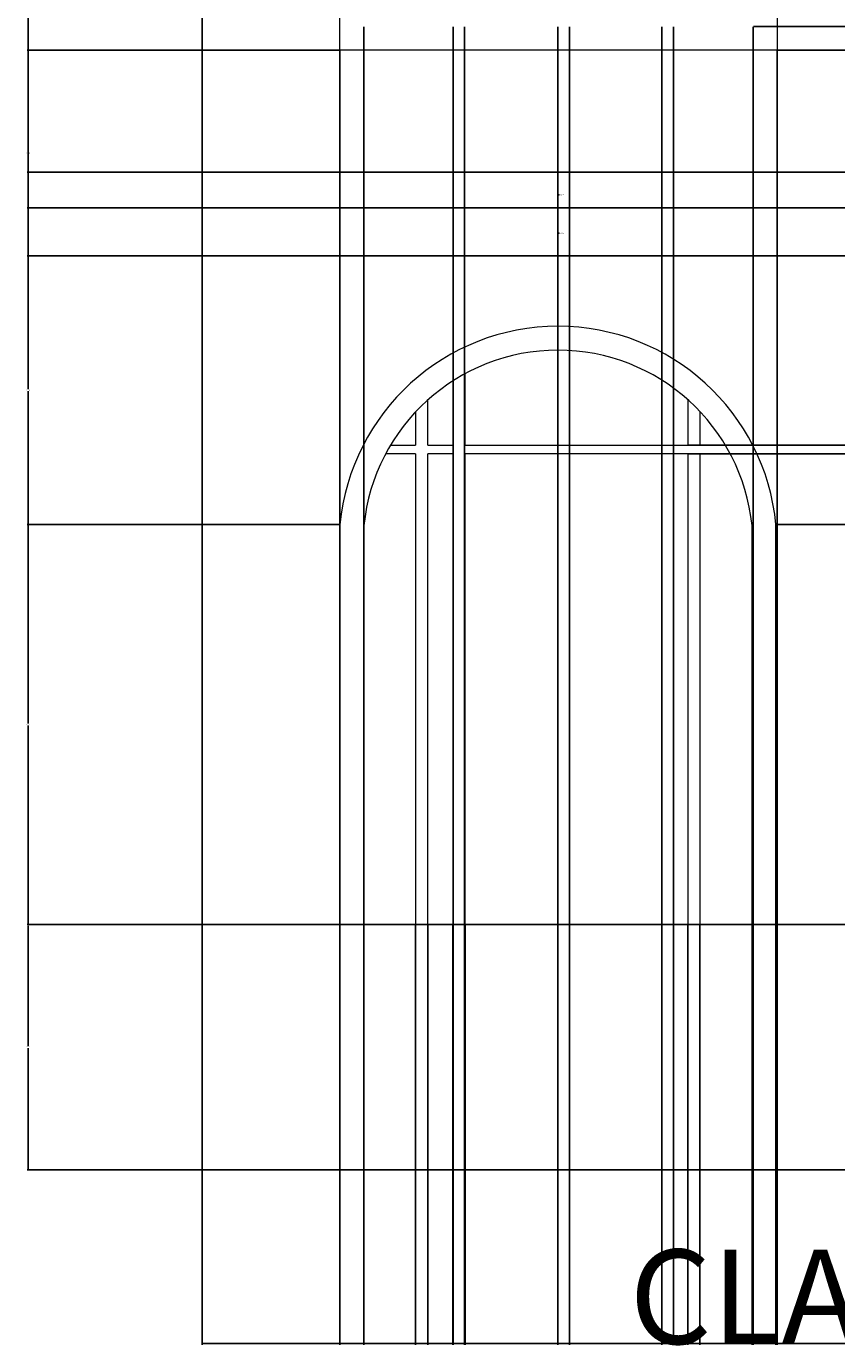
# Model space of a CAD drawing. Units: inches. Extents: x -14 to 375, y -86 to 549.
# Tile 1 of 12: x -14 to 122, y -65 to 156. Entities that reach past the tile are written whole.
import ezdxf

# ---------------------------------------------------------------- set-up
doc = ezdxf.new("R2010")
doc.units = ezdxf.units.IN
doc.header["$MEASUREMENT"] = 0
for name, color, linetype, lineweight in [('A-ANNO-DIMS', 2, 'Continuous', 18), ('A-ANNO-TEXT', 7, 'Continuous', 25), ('A-ELEV', 7, 'Continuous', 25), ('A-GLAZ', 4, 'Continuous', 18)]:
    doc.layers.add(name, color=color, linetype=linetype, lineweight=lineweight)
doc.styles.get("Standard").update_dxf_attribs({"font": 'arial.ttf'})
doc.dimstyles.get("Standard").update_dxf_attribs({"dimtxt": 0.18, "dimasz": 0.18, "dimexe": 0.18, "dimexo": 0.0625, "dimgap": 0.09, "dimtad": 0, "dimtih": 1, "dimtoh": 1, "dimdec": 4, "dimzin": 0, "dimdsep": 46, "dimtxsty": 'Standard', "dimcen": 0.09, "dimadec": 0, "dimazin": 0, "dimtfac": 1, "dimtdec": 4, "dimtofl": 0, "dimtmove": 0, "dimatfit": 3, "dimfxl": 1, "dimtolj": 1, "dimtzin": 0, "dimarcsym": 0})

# ---------------------------------------------------------------- blocks, each defined once
blk = doc.blocks.new('*D4')
at = {"layer": 'A-ANNO-DIMS', "color": 0, "lineweight": -2, "transparency": 16777216}
for p, q in [((15.4, -35.17), (15.4, -64.39)), ((345.26, -35.17), (345.26, -64.39)), ((15.58, -64.21), (179.87, -64.21)), ((345.08, -64.21), (180.8, -64.21))]:
    blk.add_line(p, q, dxfattribs=at)
at = {"layer": 'A-ANNO-DIMS', "color": 0, "transparency": 16777216}
for points in [[(15.58, -64.18), (15.58, -64.24), (15.4, -64.21)], [(345.08, -64.18), (345.08, -64.24), (345.26, -64.21)]]:
    blk.add_solid(points, dxfattribs=at)
at = {"layer": 'Defpoints', "color": 0, "transparency": 16777216}
for p in [(15.4, -35.11), (345.26, -35.11), (345.26, -64.21)]:
    blk.add_point(p, dxfattribs=at)
at = {"layer": 'A-ANNO-DIMS', "color": 0, "transparency": 16777216, "insert": (180.33, -64.21), "char_height": 0.18, "attachment_point": 5}
blk.add_mtext('\\A1;329.86', dxfattribs=at)
blk = doc.blocks.new('*D11')
at = {"layer": 'A-ANNO-DIMS', "color": 0, "lineweight": -2, "transparency": 16777216}
for p, q in [((38.44, 5.96), (-13.88, 5.96)), ((-13.7, 5.78), (-13.7, -14.39)), ((-13.7, -34.93), (-13.7, -14.76)), ((15.34, -35.11), (-13.88, -35.11))]:
    blk.add_line(p, q, dxfattribs=at)
at = {"layer": 'A-ANNO-DIMS', "color": 0, "transparency": 16777216}
for points in [[(-13.73, 5.78), (-13.67, 5.78), (-13.7, 5.96)], [(-13.73, -34.93), (-13.67, -34.93), (-13.7, -35.11)]]:
    blk.add_solid(points, dxfattribs=at)
at = {"layer": 'Defpoints', "color": 0, "transparency": 16777216}
for p in [(-13.7, 5.96), (38.5, 5.96), (15.4, -35.11)]:
    blk.add_point(p, dxfattribs=at)
at = {"layer": 'A-ANNO-DIMS', "color": 0, "transparency": 16777216, "insert": (-13.7, -14.58), "char_height": 0.18, "attachment_point": 5}
blk.add_mtext('\\A1;41.07', dxfattribs=at)
blk = doc.blocks.new('*D12')
at = {"layer": 'A-ANNO-DIMS', "color": 0, "lineweight": -2, "transparency": 16777216}
for p, q in [((38.44, 72.97), (-13.88, 72.97)), ((-13.7, 72.79), (-13.7, 39.65)), ((-13.7, 6.14), (-13.7, 39.28)), ((38.44, 5.96), (-13.88, 5.96))]:
    blk.add_line(p, q, dxfattribs=at)
at = {"layer": 'A-ANNO-DIMS', "color": 0, "transparency": 16777216}
for points in [[(-13.73, 72.79), (-13.67, 72.79), (-13.7, 72.97)], [(-13.73, 6.14), (-13.67, 6.14), (-13.7, 5.96)]]:
    blk.add_solid(points, dxfattribs=at)
at = {"layer": 'Defpoints', "color": 0, "transparency": 16777216}
for p in [(-13.7, 72.97), (38.5, 72.97), (38.5, 5.96)]:
    blk.add_point(p, dxfattribs=at)
at = {"layer": 'A-ANNO-DIMS', "color": 0, "transparency": 16777216, "insert": (-13.7, 39.46), "char_height": 0.18, "attachment_point": 5}
blk.add_mtext('\\A1;67.01', dxfattribs=at)
blk = doc.blocks.new('*D13')
at = {"layer": 'A-ANNO-DIMS', "color": 0, "lineweight": -2, "transparency": 16777216}
for p, q in [((134.17, 117.96), (-13.88, 117.96)), ((-13.7, 117.78), (-13.7, 95.65)), ((-13.7, 73.15), (-13.7, 95.28)), ((38.44, 72.97), (-13.88, 72.97))]:
    blk.add_line(p, q, dxfattribs=at)
at = {"layer": 'A-ANNO-DIMS', "color": 0, "transparency": 16777216}
for points in [[(-13.73, 117.78), (-13.67, 117.78), (-13.7, 117.96)], [(-13.73, 73.15), (-13.67, 73.15), (-13.7, 72.97)]]:
    blk.add_solid(points, dxfattribs=at)
at = {"layer": 'Defpoints', "color": 0, "transparency": 16777216}
for p in [(-13.7, 117.96), (134.23, 117.96), (38.5, 72.97)]:
    blk.add_point(p, dxfattribs=at)
at = {"layer": 'A-ANNO-DIMS', "color": 0, "transparency": 16777216, "insert": (-13.7, 95.46), "char_height": 0.18, "attachment_point": 5}
blk.add_mtext('\\A1;44.99', dxfattribs=at)
blk = doc.blocks.new('*D14')
at = {"layer": 'A-ANNO-DIMS', "color": 0, "lineweight": -2, "transparency": 16777216}
for p, q in [((38.44, 152.38), (-13.88, 152.38)), ((-13.7, 152.2), (-13.7, 135.35)), ((-13.7, 118.14), (-13.7, 134.99)), ((134.17, 117.96), (-13.88, 117.96))]:
    blk.add_line(p, q, dxfattribs=at)
at = {"layer": 'A-ANNO-DIMS', "color": 0, "transparency": 16777216}
for points in [[(-13.73, 152.2), (-13.67, 152.2), (-13.7, 152.38)], [(-13.73, 118.14), (-13.67, 118.14), (-13.7, 117.96)]]:
    blk.add_solid(points, dxfattribs=at)
at = {"layer": 'Defpoints', "color": 0, "transparency": 16777216}
for p in [(-13.7, 152.38), (38.5, 152.38), (134.23, 117.96)]:
    blk.add_point(p, dxfattribs=at)
at = {"layer": 'A-ANNO-DIMS', "color": 0, "transparency": 16777216, "insert": (-13.7, 135.17), "char_height": 0.18, "attachment_point": 5}
blk.add_mtext('\\A1;34.42', dxfattribs=at)
blk = doc.blocks.new('*D15')
at = {"layer": 'A-ANNO-DIMS', "color": 0, "lineweight": -2, "transparency": 16777216}
for p, q in [((134.17, 187.85), (-13.88, 187.85)), ((-13.7, 187.67), (-13.7, 170.29)), ((-13.7, 152.56), (-13.7, 169.93)), ((38.44, 152.38), (-13.88, 152.38))]:
    blk.add_line(p, q, dxfattribs=at)
at = {"layer": 'A-ANNO-DIMS', "color": 0, "transparency": 16777216}
for points in [[(-13.73, 187.67), (-13.67, 187.67), (-13.7, 187.85)], [(-13.73, 152.56), (-13.67, 152.56), (-13.7, 152.38)]]:
    blk.add_solid(points, dxfattribs=at)
at = {"layer": 'Defpoints', "color": 0, "transparency": 16777216}
for p in [(-13.7, 187.85), (134.23, 187.85), (38.5, 152.38)]:
    blk.add_point(p, dxfattribs=at)
at = {"layer": 'A-ANNO-DIMS', "color": 0, "transparency": 16777216, "insert": (-13.7, 170.11), "char_height": 0.18, "attachment_point": 5}
blk.add_mtext('\\A1;35.47', dxfattribs=at)
blk = doc.blocks.new('*D19')
at = {"layer": 'A-ANNO-DIMS', "color": 0, "lineweight": -2, "transparency": 16777216}
for p, q in [((42.5, 156.31), (42.5, -64.39)), ((38.5, 152.31), (38.5, -64.39)), ((38.68, -64.21), (40.35, -64.21)), ((42.32, -64.21), (40.66, -64.21))]:
    blk.add_line(p, q, dxfattribs=at)
at = {"layer": 'A-ANNO-DIMS', "color": 0, "transparency": 16777216}
for points in [[(38.68, -64.18), (38.68, -64.24), (38.5, -64.21)], [(42.32, -64.18), (42.32, -64.24), (42.5, -64.21)]]:
    blk.add_solid(points, dxfattribs=at)
at = {"layer": 'Defpoints', "color": 0, "transparency": 16777216}
for p in [(42.5, 156.38), (38.5, 152.38), (42.5, -64.21)]:
    blk.add_point(p, dxfattribs=at)
at = {"layer": 'A-ANNO-DIMS', "color": 0, "transparency": 16777216, "insert": (40.5, -64.21), "char_height": 0.18, "attachment_point": 5}
blk.add_mtext('\\A1;4', dxfattribs=at)
blk = doc.blocks.new('*D20')
at = {"layer": 'A-ANNO-DIMS', "color": 0, "lineweight": -2, "transparency": 16777216}
for p, q in [((42.5, 156.31), (42.5, -64.39)), ((57.44, 156.31), (57.44, -64.39)), ((42.68, -64.21), (49.52, -64.21)), ((57.26, -64.21), (50.43, -64.21))]:
    blk.add_line(p, q, dxfattribs=at)
at = {"layer": 'A-ANNO-DIMS', "color": 0, "transparency": 16777216}
for points in [[(42.68, -64.18), (42.68, -64.24), (42.5, -64.21)], [(57.26, -64.18), (57.26, -64.24), (57.44, -64.21)]]:
    blk.add_solid(points, dxfattribs=at)
at = {"layer": 'Defpoints', "color": 0, "transparency": 16777216}
for p in [(42.5, 156.38), (57.44, 156.38), (57.44, -64.21)]:
    blk.add_point(p, dxfattribs=at)
at = {"layer": 'A-ANNO-DIMS', "color": 0, "transparency": 16777216, "insert": (49.97, -64.21), "char_height": 0.18, "attachment_point": 5}
blk.add_mtext('\\A1;14.938', dxfattribs=at)
blk = doc.blocks.new('*D21')
at = {"layer": 'A-ANNO-DIMS', "color": 0, "lineweight": -2, "transparency": 16777216}
for p, q in [((57.44, 156.31), (57.44, -64.39)), ((59.36, 156.31), (59.36, -64.39)), ((57.62, -64.21), (58.09, -64.21)), ((59.18, -64.21), (58.72, -64.21))]:
    blk.add_line(p, q, dxfattribs=at)
at = {"layer": 'A-ANNO-DIMS', "color": 0, "transparency": 16777216}
for points in [[(57.62, -64.18), (57.62, -64.24), (57.44, -64.21)], [(59.18, -64.18), (59.18, -64.24), (59.36, -64.21)]]:
    blk.add_solid(points, dxfattribs=at)
at = {"layer": 'Defpoints', "color": 0, "transparency": 16777216}
for p in [(57.44, 156.38), (59.36, 156.38), (59.36, -64.21)]:
    blk.add_point(p, dxfattribs=at)
at = {"layer": 'A-ANNO-DIMS', "color": 0, "transparency": 16777216, "insert": (58.4, -64.21), "char_height": 0.18, "attachment_point": 5}
blk.add_mtext('\\A1;1.92', dxfattribs=at)
blk = doc.blocks.new('*D22')
at = {"layer": 'A-ANNO-DIMS', "color": 0, "lineweight": -2, "transparency": 16777216}
for p, q in [((59.36, 156.31), (59.36, -64.39)), ((75, 156.31), (75, -64.39)), ((59.54, -64.21), (66.73, -64.21)), ((74.82, -64.21), (67.64, -64.21))]:
    blk.add_line(p, q, dxfattribs=at)
at = {"layer": 'A-ANNO-DIMS', "color": 0, "transparency": 16777216}
for points in [[(59.54, -64.18), (59.54, -64.24), (59.36, -64.21)], [(74.82, -64.18), (74.82, -64.24), (75, -64.21)]]:
    blk.add_solid(points, dxfattribs=at)
at = {"layer": 'Defpoints', "color": 0, "transparency": 16777216}
for p in [(59.36, 156.38), (75, 156.38), (75, -64.21)]:
    blk.add_point(p, dxfattribs=at)
at = {"layer": 'A-ANNO-DIMS', "color": 0, "transparency": 16777216, "insert": (67.18, -64.21), "char_height": 0.18, "attachment_point": 5}
blk.add_mtext('\\A1;15.637', dxfattribs=at)
blk = doc.blocks.new('*D23')
at = {"layer": 'A-ANNO-DIMS', "color": 0, "lineweight": -2, "transparency": 16777216}
for p, q in [((75, 156.31), (75, -64.39)), ((76.92, 156.31), (76.92, -64.39)), ((75.18, -64.21), (75.65, -64.21)), ((76.74, -64.21), (76.28, -64.21))]:
    blk.add_line(p, q, dxfattribs=at)
at = {"layer": 'A-ANNO-DIMS', "color": 0, "transparency": 16777216}
for points in [[(75.18, -64.18), (75.18, -64.24), (75, -64.21)], [(76.74, -64.18), (76.74, -64.24), (76.92, -64.21)]]:
    blk.add_solid(points, dxfattribs=at)
at = {"layer": 'Defpoints', "color": 0, "transparency": 16777216}
for p in [(75, 156.38), (76.92, 156.38), (76.92, -64.21)]:
    blk.add_point(p, dxfattribs=at)
at = {"layer": 'A-ANNO-DIMS', "color": 0, "transparency": 16777216, "insert": (75.96, -64.21), "char_height": 0.18, "attachment_point": 5}
blk.add_mtext('\\A1;1.92', dxfattribs=at)
blk = doc.blocks.new('*D24')
at = {"layer": 'A-ANNO-DIMS', "color": 0, "lineweight": -2, "transparency": 16777216}
for p, q in [((76.92, 156.31), (76.92, -64.39)), ((92.4, 156.31), (92.4, -64.39)), ((77.1, -64.21), (84.2, -64.21)), ((92.22, -64.21), (85.12, -64.21))]:
    blk.add_line(p, q, dxfattribs=at)
at = {"layer": 'A-ANNO-DIMS', "color": 0, "transparency": 16777216}
for points in [[(77.1, -64.18), (77.1, -64.24), (76.92, -64.21)], [(92.22, -64.18), (92.22, -64.24), (92.4, -64.21)]]:
    blk.add_solid(points, dxfattribs=at)
at = {"layer": 'Defpoints', "color": 0, "transparency": 16777216}
for p in [(76.92, 156.38), (92.4, 156.38), (92.4, -64.21)]:
    blk.add_point(p, dxfattribs=at)
at = {"layer": 'A-ANNO-DIMS', "color": 0, "transparency": 16777216, "insert": (84.66, -64.21), "char_height": 0.18, "attachment_point": 5}
blk.add_mtext('\\A1;15.473', dxfattribs=at)
blk = doc.blocks.new('*D25')
at = {"layer": 'A-ANNO-DIMS', "color": 0, "lineweight": -2, "transparency": 16777216}
for p, q in [((92.4, 156.31), (92.4, -64.39)), ((94.32, 156.31), (94.32, -64.39)), ((92.58, -64.21), (93.04, -64.21)), ((94.14, -64.21), (93.67, -64.21))]:
    blk.add_line(p, q, dxfattribs=at)
at = {"layer": 'A-ANNO-DIMS', "color": 0, "transparency": 16777216}
for points in [[(92.58, -64.18), (92.58, -64.24), (92.4, -64.21)], [(94.14, -64.18), (94.14, -64.24), (94.32, -64.21)]]:
    blk.add_solid(points, dxfattribs=at)
at = {"layer": 'Defpoints', "color": 0, "transparency": 16777216}
for p in [(92.4, 156.38), (94.32, 156.38), (94.32, -64.21)]:
    blk.add_point(p, dxfattribs=at)
at = {"layer": 'A-ANNO-DIMS', "color": 0, "transparency": 16777216, "insert": (93.36, -64.21), "char_height": 0.18, "attachment_point": 5}
blk.add_mtext('\\A1;1.92', dxfattribs=at)
blk = doc.blocks.new('*D26')
at = {"layer": 'A-ANNO-DIMS', "color": 0, "lineweight": -2, "transparency": 16777216}
for p, q in [((94.32, 156.31), (94.32, -64.39)), ((107.7, 156.31), (107.7, -64.39)), ((94.5, -64.21), (100.56, -64.21)), ((107.52, -64.21), (101.47, -64.21))]:
    blk.add_line(p, q, dxfattribs=at)
at = {"layer": 'A-ANNO-DIMS', "color": 0, "transparency": 16777216}
for points in [[(94.5, -64.18), (94.5, -64.24), (94.32, -64.21)], [(107.52, -64.18), (107.52, -64.24), (107.7, -64.21)]]:
    blk.add_solid(points, dxfattribs=at)
at = {"layer": 'Defpoints', "color": 0, "transparency": 16777216}
for p in [(94.32, 156.38), (107.7, 156.38), (107.7, -64.21)]:
    blk.add_point(p, dxfattribs=at)
at = {"layer": 'A-ANNO-DIMS', "color": 0, "transparency": 16777216, "insert": (101.01, -64.21), "char_height": 0.18, "attachment_point": 5}
blk.add_mtext('\\A1;13.383', dxfattribs=at)
blk = doc.blocks.new('*D27')
at = {"layer": 'A-ANNO-DIMS', "color": 0, "lineweight": -2, "transparency": 16777216}
for p, q in [((107.7, 156.31), (107.7, -64.39)), ((111.7, 152.31), (111.7, -64.39)), ((107.88, -64.21), (109.55, -64.21)), ((111.52, -64.21), (109.85, -64.21))]:
    blk.add_line(p, q, dxfattribs=at)
at = {"layer": 'A-ANNO-DIMS', "color": 0, "transparency": 16777216}
for points in [[(107.88, -64.18), (107.88, -64.24), (107.7, -64.21)], [(111.52, -64.18), (111.52, -64.24), (111.7, -64.21)]]:
    blk.add_solid(points, dxfattribs=at)
at = {"layer": 'Defpoints', "color": 0, "transparency": 16777216}
for p in [(107.7, 156.38), (111.7, 152.38), (111.7, -64.21)]:
    blk.add_point(p, dxfattribs=at)
at = {"layer": 'A-ANNO-DIMS', "color": 0, "transparency": 16777216, "insert": (109.7, -64.21), "char_height": 0.18, "attachment_point": 5}
blk.add_mtext('\\A1;4', dxfattribs=at)
blk = doc.blocks.new('*D28')
at = {"layer": 'A-ANNO-DIMS', "color": 0, "lineweight": -2, "transparency": 16777216}
for p, q in [((107.764387, 156.376775), (374.544714, 156.376775)), ((374.364714, 156.196775), (374.364714, 154.556775)), ((374.364714, 152.556775), (374.364714, 154.196775)), ((111.764387, 152.376775), (374.544714, 152.376775))]:
    blk.add_line(p, q, dxfattribs=at)
at = {"layer": 'A-ANNO-DIMS', "color": 0, "transparency": 16777216}
for points in [[(374.334714, 156.196775), (374.394714, 156.196775), (374.364714, 156.376775)], [(374.334714, 152.556775), (374.394714, 152.556775), (374.364714, 152.376775)]]:
    blk.add_solid(points, dxfattribs=at)
at = {"layer": 'Defpoints', "color": 0, "transparency": 16777216}
for p in [(107.701887, 156.376775), (374.364714, 156.376775), (111.701887, 152.376775)]:
    blk.add_point(p, dxfattribs=at)
at = {"layer": 'A-ANNO-DIMS', "color": 0, "transparency": 16777216, "insert": (374.364714, 154.376775), "char_height": 0.18, "attachment_point": 5}
blk.add_mtext('\\A1;4', dxfattribs=at)
blk = doc.blocks.new('*D29')
at = {"layer": 'A-ANNO-DIMS', "color": 0, "lineweight": -2, "transparency": 16777216}
for p, q in [((107.74, 193.48), (374.54, 193.48)), ((374.36, 193.3), (374.36, 175.11)), ((374.36, 156.56), (374.36, 174.75)), ((107.76, 156.38), (374.54, 156.38))]:
    blk.add_line(p, q, dxfattribs=at)
at = {"layer": 'A-ANNO-DIMS', "color": 0, "transparency": 16777216}
for points in [[(374.33, 193.3), (374.39, 193.3), (374.36, 193.48)], [(374.33, 156.56), (374.39, 156.56), (374.36, 156.38)]]:
    blk.add_solid(points, dxfattribs=at)
at = {"layer": 'Defpoints', "color": 0, "transparency": 16777216}
for p in [(107.68, 193.48), (374.36, 193.48), (107.7, 156.38)]:
    blk.add_point(p, dxfattribs=at)
at = {"layer": 'A-ANNO-DIMS', "color": 0, "transparency": 16777216, "insert": (374.36, 174.93), "char_height": 0.18, "attachment_point": 5}
blk.add_mtext('\\A1;37.106', dxfattribs=at)
blk = doc.blocks.new('*D95')
at = {"layer": 'A-ANNO-DIMS', "color": 0, "lineweight": -2, "transparency": 16777216}
for p, q in [((194.3, 131.97), (-13.88, 131.97)), ((-13.7, 131.79), (-13.7, 129.15)), ((-13.7, 126.15), (-13.7, 128.79)), ((187.3, 125.97), (-13.88, 125.97))]:
    blk.add_line(p, q, dxfattribs=at)
at = {"layer": 'A-ANNO-DIMS', "color": 0, "transparency": 16777216}
for points in [[(-13.73, 131.79), (-13.67, 131.79), (-13.7, 131.97)], [(-13.73, 126.15), (-13.67, 126.15), (-13.7, 125.97)]]:
    blk.add_solid(points, dxfattribs=at)
at = {"layer": 'Defpoints', "color": 0, "transparency": 16777216}
for p in [(-13.7, 131.97), (194.37, 131.97), (187.37, 125.97)]:
    blk.add_point(p, dxfattribs=at)
at = {"layer": 'A-ANNO-DIMS', "color": 0, "transparency": 16777216, "insert": (-13.7, 128.97), "char_height": 0.18, "attachment_point": 5}
blk.add_mtext('\\A1;6', dxfattribs=at)
blk = doc.blocks.new('*D96')
at = {"layer": 'A-ANNO-DIMS', "color": 0, "lineweight": -2, "transparency": 16777216}
for p, q in [((194.3, 200.95), (-13.88, 200.95)), ((-13.7, 200.77), (-13.7, 166.64)), ((-13.7, 132.15), (-13.7, 166.28)), ((194.3, 131.97), (-13.88, 131.97))]:
    blk.add_line(p, q, dxfattribs=at)
at = {"layer": 'A-ANNO-DIMS', "color": 0, "transparency": 16777216}
for points in [[(-13.73, 200.77), (-13.67, 200.77), (-13.7, 200.95)], [(-13.73, 132.15), (-13.67, 132.15), (-13.7, 131.97)]]:
    blk.add_solid(points, dxfattribs=at)
at = {"layer": 'Defpoints', "color": 0, "transparency": 16777216}
for p in [(-13.7, 200.95), (194.37, 200.95), (194.37, 131.97)]:
    blk.add_point(p, dxfattribs=at)
at = {"layer": 'A-ANNO-DIMS', "color": 0, "transparency": 16777216, "insert": (-13.7, 166.46), "char_height": 0.18, "attachment_point": 5}
blk.add_mtext('\\A1;68.98', dxfattribs=at)
blk = doc.blocks.new('*D119')
at = {"layer": 'A-ANNO-DIMS', "color": 0, "lineweight": -2, "transparency": 16777216}
for p, q in [((38.5, 5.9), (38.5, -64.39)), ((42.5, 5.9), (42.5, -64.39)), ((38.68, -64.21), (40.35, -64.21)), ((42.32, -64.21), (40.66, -64.21))]:
    blk.add_line(p, q, dxfattribs=at)
at = {"layer": 'A-ANNO-DIMS', "color": 0, "transparency": 16777216}
for points in [[(38.68, -64.18), (38.68, -64.24), (38.5, -64.21)], [(42.32, -64.18), (42.32, -64.24), (42.5, -64.21)]]:
    blk.add_solid(points, dxfattribs=at)
at = {"layer": 'Defpoints', "color": 0, "transparency": 16777216}
for p in [(38.5, 5.96), (42.5, 5.96), (42.5, -64.21)]:
    blk.add_point(p, dxfattribs=at)
at = {"layer": 'A-ANNO-DIMS', "color": 0, "transparency": 16777216, "insert": (40.5, -64.21), "char_height": 0.18, "attachment_point": 5}
blk.add_mtext('\\A1;4', dxfattribs=at)
blk = doc.blocks.new('*D120')
at = {"layer": 'A-ANNO-DIMS', "color": 0, "lineweight": -2, "transparency": 16777216}
for p, q in [((42.5, 5.9), (42.5, -64.39)), ((51.16, 5.9), (51.16, -64.39)), ((42.68, -64.21), (46.51, -64.21)), ((50.98, -64.21), (47.16, -64.21))]:
    blk.add_line(p, q, dxfattribs=at)
at = {"layer": 'A-ANNO-DIMS', "color": 0, "transparency": 16777216}
for points in [[(42.68, -64.18), (42.68, -64.24), (42.5, -64.21)], [(50.98, -64.18), (50.98, -64.24), (51.16, -64.21)]]:
    blk.add_solid(points, dxfattribs=at)
at = {"layer": 'Defpoints', "color": 0, "transparency": 16777216}
for p in [(42.5, 5.96), (51.16, 5.96), (51.16, -64.21)]:
    blk.add_point(p, dxfattribs=at)
at = {"layer": 'A-ANNO-DIMS', "color": 0, "transparency": 16777216, "insert": (46.83, -64.21), "char_height": 0.18, "attachment_point": 5}
blk.add_mtext('\\A1;8.66', dxfattribs=at)
blk = doc.blocks.new('*D121')
at = {"layer": 'A-ANNO-DIMS', "color": 0, "lineweight": -2, "transparency": 16777216}
for p, q in [((51.16, 5.9), (51.16, -64.39)), ((53.22, 5.9), (53.22, -64.39)), ((51.34, -64.21), (51.87, -64.21)), ((53.04, -64.21), (52.52, -64.21))]:
    blk.add_line(p, q, dxfattribs=at)
at = {"layer": 'A-ANNO-DIMS', "color": 0, "transparency": 16777216}
for points in [[(51.34, -64.18), (51.34, -64.24), (51.16, -64.21)], [(53.04, -64.18), (53.04, -64.24), (53.22, -64.21)]]:
    blk.add_solid(points, dxfattribs=at)
at = {"layer": 'Defpoints', "color": 0, "transparency": 16777216}
for p in [(51.16, 5.96), (53.22, 5.96), (53.22, -64.21)]:
    blk.add_point(p, dxfattribs=at)
at = {"layer": 'A-ANNO-DIMS', "color": 0, "transparency": 16777216, "insert": (52.19, -64.21), "char_height": 0.18, "attachment_point": 5}
blk.add_mtext('\\A1;2.06', dxfattribs=at)
blk = doc.blocks.new('*D122')
at = {"layer": 'A-ANNO-DIMS', "color": 0, "lineweight": -2, "transparency": 16777216}
for p, q in [((53.22, 5.9), (53.22, -64.39)), ((57.38, 5.9), (57.38, -64.39)), ((53.4, -64.21), (54.9, -64.21)), ((57.2, -64.21), (55.7, -64.21))]:
    blk.add_line(p, q, dxfattribs=at)
at = {"layer": 'A-ANNO-DIMS', "color": 0, "transparency": 16777216}
for points in [[(53.4, -64.18), (53.4, -64.24), (53.22, -64.21)], [(57.2, -64.18), (57.2, -64.24), (57.38, -64.21)]]:
    blk.add_solid(points, dxfattribs=at)
at = {"layer": 'Defpoints', "color": 0, "transparency": 16777216}
for p in [(53.22, 5.96), (57.38, 5.96), (57.38, -64.21)]:
    blk.add_point(p, dxfattribs=at)
at = {"layer": 'A-ANNO-DIMS', "color": 0, "transparency": 16777216, "insert": (55.3, -64.21), "char_height": 0.18, "attachment_point": 5}
blk.add_mtext('\\A1;4.158', dxfattribs=at)
blk = doc.blocks.new('*D123')
at = {"layer": 'A-ANNO-DIMS', "color": 0, "lineweight": -2, "transparency": 16777216}
for p, q in [((57.38, 5.9), (57.38, -64.39)), ((59.44, 5.9), (59.44, -64.39)), ((57.56, -64.21), (58.08, -64.21)), ((59.26, -64.21), (58.73, -64.21))]:
    blk.add_line(p, q, dxfattribs=at)
at = {"layer": 'A-ANNO-DIMS', "color": 0, "transparency": 16777216}
for points in [[(57.56, -64.18), (57.56, -64.24), (57.38, -64.21)], [(59.26, -64.18), (59.26, -64.24), (59.44, -64.21)]]:
    blk.add_solid(points, dxfattribs=at)
at = {"layer": 'Defpoints', "color": 0, "transparency": 16777216}
for p in [(57.38, 5.96), (59.44, 5.96), (59.44, -64.21)]:
    blk.add_point(p, dxfattribs=at)
at = {"layer": 'A-ANNO-DIMS', "color": 0, "transparency": 16777216, "insert": (58.41, -64.21), "char_height": 0.18, "attachment_point": 5}
blk.add_mtext('\\A1;2.06', dxfattribs=at)
blk = doc.blocks.new('*D124')
at = {"layer": 'A-ANNO-DIMS', "color": 0, "lineweight": -2, "transparency": 16777216}
for p, q in [((59.44, 5.9), (59.44, -64.39)), ((96.73, 5.9), (96.73, -64.39)), ((59.62, -64.21), (77.69, -64.21)), ((96.55, -64.21), (78.48, -64.21))]:
    blk.add_line(p, q, dxfattribs=at)
at = {"layer": 'A-ANNO-DIMS', "color": 0, "transparency": 16777216}
for points in [[(59.62, -64.18), (59.62, -64.24), (59.44, -64.21)], [(96.55, -64.18), (96.55, -64.24), (96.73, -64.21)]]:
    blk.add_solid(points, dxfattribs=at)
at = {"layer": 'Defpoints', "color": 0, "transparency": 16777216}
for p in [(59.44, 5.96), (96.73, 5.96), (96.73, -64.21)]:
    blk.add_point(p, dxfattribs=at)
at = {"layer": 'A-ANNO-DIMS', "color": 0, "transparency": 16777216, "insert": (78.08, -64.21), "char_height": 0.18, "attachment_point": 5}
blk.add_mtext('\\A1;37.29', dxfattribs=at)
blk = doc.blocks.new('*D125')
at = {"layer": 'A-ANNO-DIMS', "color": 0, "lineweight": -2, "transparency": 16777216}
for p, q in [((96.73, 5.9), (96.73, -64.39)), ((98.78, 5.9), (98.78, -64.39)), ((96.91, -64.21), (97.43, -64.21)), ((98.6, -64.21), (98.08, -64.21))]:
    blk.add_line(p, q, dxfattribs=at)
at = {"layer": 'A-ANNO-DIMS', "color": 0, "transparency": 16777216}
for points in [[(96.91, -64.18), (96.91, -64.24), (96.73, -64.21)], [(98.6, -64.18), (98.6, -64.24), (98.78, -64.21)]]:
    blk.add_solid(points, dxfattribs=at)
at = {"layer": 'Defpoints', "color": 0, "transparency": 16777216}
for p in [(96.73, 5.96), (98.78, 5.96), (98.78, -64.21)]:
    blk.add_point(p, dxfattribs=at)
at = {"layer": 'A-ANNO-DIMS', "color": 0, "transparency": 16777216, "insert": (97.75, -64.21), "char_height": 0.18, "attachment_point": 5}
blk.add_mtext('\\A1;2.06', dxfattribs=at)
blk = doc.blocks.new('*D126')
at = {"layer": 'A-ANNO-DIMS', "color": 0, "lineweight": -2, "transparency": 16777216}
for p, q in [((98.78, 5.9), (98.78, -64.39)), ((107.5, 5.9), (107.5, -64.39)), ((98.96, -64.21), (102.75, -64.21)), ((107.32, -64.21), (103.54, -64.21))]:
    blk.add_line(p, q, dxfattribs=at)
at = {"layer": 'A-ANNO-DIMS', "color": 0, "transparency": 16777216}
for points in [[(98.96, -64.18), (98.96, -64.24), (98.78, -64.21)], [(107.32, -64.18), (107.32, -64.24), (107.5, -64.21)]]:
    blk.add_solid(points, dxfattribs=at)
at = {"layer": 'Defpoints', "color": 0, "transparency": 16777216}
for p in [(98.78, 5.96), (107.5, 5.96), (107.5, -64.21)]:
    blk.add_point(p, dxfattribs=at)
at = {"layer": 'A-ANNO-DIMS', "color": 0, "transparency": 16777216, "insert": (103.14, -64.21), "char_height": 0.18, "attachment_point": 5}
blk.add_mtext('\\A1;8.715', dxfattribs=at)
blk = doc.blocks.new('*D127')
at = {"layer": 'A-ANNO-DIMS', "color": 0, "lineweight": -2, "transparency": 16777216}
for p, q in [((107.5, 5.9), (107.5, -64.39)), ((111.5, 5.9), (111.5, -64.39)), ((107.68, -64.21), (109.35, -64.21)), ((111.32, -64.21), (109.65, -64.21))]:
    blk.add_line(p, q, dxfattribs=at)
at = {"layer": 'A-ANNO-DIMS', "color": 0, "transparency": 16777216}
for points in [[(107.68, -64.18), (107.68, -64.24), (107.5, -64.21)], [(111.32, -64.18), (111.32, -64.24), (111.5, -64.21)]]:
    blk.add_solid(points, dxfattribs=at)
at = {"layer": 'Defpoints', "color": 0, "transparency": 16777216}
for p in [(107.5, 5.96), (111.5, 5.96), (111.5, -64.21)]:
    blk.add_point(p, dxfattribs=at)
at = {"layer": 'A-ANNO-DIMS', "color": 0, "transparency": 16777216, "insert": (109.5, -64.21), "char_height": 0.18, "attachment_point": 5}
blk.add_mtext('\\A1;4', dxfattribs=at)
blk = doc.blocks.new('*D128')
at = {"layer": 'A-ANNO-DIMS', "color": 0, "lineweight": -2, "transparency": 16777216}
for p, q in [((96.79, 84.82), (374.54, 84.82)), ((374.36, 84.64), (374.36, 79.07)), ((374.36, 73.15), (374.36, 78.71)), ((111.56, 72.97), (374.54, 72.97))]:
    blk.add_line(p, q, dxfattribs=at)
at = {"layer": 'A-ANNO-DIMS', "color": 0, "transparency": 16777216}
for points in [[(374.33, 84.64), (374.39, 84.64), (374.36, 84.82)], [(374.33, 73.15), (374.39, 73.15), (374.36, 72.97)]]:
    blk.add_solid(points, dxfattribs=at)
at = {"layer": 'Defpoints', "color": 0, "transparency": 16777216}
for p in [(96.73, 84.82), (374.36, 84.82), (111.5, 72.97)]:
    blk.add_point(p, dxfattribs=at)
at = {"layer": 'A-ANNO-DIMS', "color": 0, "transparency": 16777216, "insert": (374.36, 78.89), "char_height": 0.18, "attachment_point": 5}
blk.add_mtext('\\A1;11.849', dxfattribs=at)
blk = doc.blocks.new('*D129')
at = {"layer": 'A-ANNO-DIMS', "color": 0, "lineweight": -2, "transparency": 16777216}
for p, q in [((96.79, 86.23), (374.54, 86.23)), ((96.79, 84.82), (374.54, 84.82)), ((374.36, 86.05), (374.36, 85.7)), ((374.36, 85), (374.36, 85.34))]:
    blk.add_line(p, q, dxfattribs=at)
at = {"layer": 'A-ANNO-DIMS', "color": 0, "transparency": 16777216}
for points in [[(374.33, 86.05), (374.39, 86.05), (374.36, 86.23)], [(374.33, 85), (374.39, 85), (374.36, 84.82)]]:
    blk.add_solid(points, dxfattribs=at)
at = {"layer": 'Defpoints', "color": 0, "transparency": 16777216}
for p in [(96.73, 86.23), (374.36, 86.23), (96.73, 84.82)]:
    blk.add_point(p, dxfattribs=at)
at = {"layer": 'A-ANNO-DIMS', "color": 0, "transparency": 16777216, "insert": (374.36, 85.52), "char_height": 0.18, "attachment_point": 5}
blk.add_mtext('\\A1;1.409', dxfattribs=at)
blk = doc.blocks.new('*D139')
at = {"layer": 'A-ANNO-DIMS', "color": 0, "lineweight": -2, "transparency": 16777216}
for p, q in [((75.18, 128.15), (75, 128.15)), ((75, 128.15), (75, 106.33)), ((74.91, 69.49), (75.09, 69.49)), ((75, 69.4), (75, 69.58))]:
    blk.add_line(p, q, dxfattribs=at)
at = {"layer": 'A-ANNO-DIMS', "color": 0, "transparency": 16777216}
blk.add_solid([(74.97, 106.33), (75.03, 106.33), (75, 106.15)], dxfattribs=at)
at = {"layer": 'Defpoints', "color": 0, "transparency": 16777216}
for p in [(75, 106.15), (75, 69.49)]:
    blk.add_point(p, dxfattribs=at)
at = {"layer": 'A-ANNO-DIMS', "color": 0, "transparency": 16777216, "insert": (75.66, 128.15), "char_height": 0.18, "attachment_point": 5}
blk.add_mtext('\\A1;R36.66', dxfattribs=at)
blk = doc.blocks.new('*D140')
at = {"layer": 'A-ANNO-DIMS', "color": 0, "lineweight": -2, "transparency": 16777216}
for p, q in [((75.18, 121.75), (75, 121.75)), ((75, 121.75), (75, 102.33)), ((74.91, 69.49), (75.09, 69.49)), ((75, 69.4), (75, 69.58))]:
    blk.add_line(p, q, dxfattribs=at)
at = {"layer": 'A-ANNO-DIMS', "color": 0, "transparency": 16777216}
blk.add_solid([(74.97, 102.33), (75.03, 102.33), (75, 102.15)], dxfattribs=at)
at = {"layer": 'Defpoints', "color": 0, "transparency": 16777216}
for p in [(75, 102.15), (75, 69.49)]:
    blk.add_point(p, dxfattribs=at)
at = {"layer": 'A-ANNO-DIMS', "color": 0, "transparency": 16777216, "insert": (75.66, 121.75), "char_height": 0.18, "attachment_point": 5}
blk.add_mtext('\\A1;R32.66', dxfattribs=at)

msp = doc.modelspace()

# ---------------------------------------------------------------- linework, layer by layer
at = {"layer": 'A-ELEV'}
for p, q in [((15.4018, 245.9589), (15.4018, 125.9589)), ((15.4018, 125.9589), (15.4018, 5.9589)), ((15.4018, 5.9589), (345.2647, 5.9589))]:
    msp.add_line(p, q, dxfattribs=at)
msp.add_lwpolyline([(15.4018, 5.9589), (345.2647, 5.9589), (345.2647, -35.1115), (15.4018, -35.1115)], close=True, dxfattribs=at)
at = {"layer": 'A-GLAZ'}
for p, q in [((46.9518, 86.2255), (51.1636, 86.2255)), ((53.222, 86.2255), (57.3803, 86.2255)), ((59.4388, 86.2255), (96.7255, 86.2255)), ((98.784, 86.2255), (103.0502, 86.2255)), ((51.1636, 84.8165), (46.1576, 84.8165)), ((57.3803, 84.8165), (53.222, 84.8165)), ((96.7255, 84.8165), (59.4388, 84.8165)), ((103.8444, 84.8165), (98.784, 84.8165))]:
    msp.add_line(p, q, dxfattribs=at)
for points in [[(111.4987, 365.9589), (111.7019, 152.3768), (38.5033, 152.3768), (38.5033, 365.9589), (38.5033, 432.9679, -0.90920588), (111.4987, 432.9679), (111.4987, 365.9589)], [(111.4987, 5.9589), (111.4987, 72.9679, 0.90920588), (38.5033, 72.9679), (38.5033, 5.9589)], [(107.4987, 5.9589), (107.4987, 72.7722, 0.9040533), (42.5033, 72.7722), (42.5033, 5.9589)]]:
    msp.add_lwpolyline(points, format="xyb", dxfattribs=at)
for points in [[(59.4388, 86.2255), (59.4388, 98.2062)], [(57.3803, 96.9913), (57.3803, 86.2255)], [(53.222, 86.2255), (53.222, 93.8312)], [(96.7255, 93.8798), (96.7255, 86.2255)], [(51.1636, 91.8193), (51.1636, 86.2255)], [(98.784, 86.2255), (98.784, 91.8773)], [(51.1636, 84.8165), (51.1636, 5.9589), (53.222, 5.9589), (53.222, 84.8165)], [(57.3803, 84.8165), (57.3803, 5.9589), (59.4388, 5.9589), (59.4388, 84.8165)], [(96.7255, 84.8165), (96.7255, 5.9589), (98.784, 5.9589), (98.784, 84.8165)]]:
    msp.add_lwpolyline(points, dxfattribs=at)

# ---------------------------------------------------------------- texts
at = {"layer": 'A-ANNO-TEXT'}
msp.add_text('CLASSIC ELEVATION', height=15.79618, dxfattribs=at).set_placement((86.9661, -64.2648))

# ---------------------------------------------------------------- dimensions: what is measured, and where the dimension line sits
at = {"layer": 'A-ANNO-DIMS'}
for base, p1, p2, override, picture, middle in [((-13.6982, 200.9487), (194.3657, 131.9717), (194.3657, 200.9487), {"dimdec": 2, "dimlfac": 1, "dimrnd": 0, "dimzin": 0, "dimdsep": 46, "dimlunit": 2}, '*D96', (-13.6982, 166.4602)), ((374.3647, 193.4825), (107.7019, 156.3768), (107.6798, 193.4825), {"dimdec": 3, "dimlfac": 1, "dimrnd": 0, "dimzin": 0, "dimdsep": 46, "dimlunit": 2}, '*D29', (374.3647, 174.9296)), ((-13.6982, 187.8466), (38.5033, 152.3768), (134.2334, 187.8466), {"dimdec": 2, "dimlfac": 1, "dimrnd": 0, "dimzin": 0, "dimdsep": 46, "dimlunit": 2}, '*D15', (-13.6982, 170.1117)), ((374.3647, 156.3768), (111.7019, 152.3768), (107.7019, 156.3768), {"dimdec": 0, "dimlfac": 1, "dimrnd": 0, "dimzin": 0, "dimdsep": 46, "dimlunit": 2}, '*D28', (374.3647, 154.3768)), ((-13.6982, 152.3768), (134.2334, 117.9589), (38.5033, 152.3768), {"dimdec": 2, "dimlfac": 1, "dimrnd": 0, "dimzin": 0, "dimdsep": 46, "dimlunit": 2}, '*D14', (-13.6982, 135.1678)), ((-13.6982, 131.9717), (187.3657, 125.9717), (194.3657, 131.9717), {"dimdec": 0, "dimlfac": 1, "dimrnd": 0, "dimzin": 0, "dimdsep": 46, "dimlunit": 2}, '*D95', (-13.6982, 128.9717)), ((-13.6982, 117.9589), (38.5033, 72.9679), (134.2334, 117.9589), {"dimdec": 2, "dimlfac": 1, "dimrnd": 0, "dimzin": 0, "dimdsep": 46, "dimlunit": 2}, '*D13', (-13.6982, 95.4634)), ((374.3647, 86.2255), (96.7255, 84.8165), (96.7255, 86.2255), {"dimdec": 3, "dimlfac": 1, "dimrnd": 0, "dimzin": 0, "dimdsep": 46, "dimlunit": 2}, '*D129', (374.3647, 85.521)), ((374.3647, 84.8165), (111.4987, 72.9679), (96.7255, 84.8165), {"dimdec": 3, "dimlfac": 1, "dimrnd": 0, "dimzin": 0, "dimdsep": 46, "dimlunit": 2}, '*D128', (374.3647, 78.8922)), ((-13.6982, 72.9679), (38.5033, 5.9589), (38.5033, 72.9679), {"dimdec": 2, "dimlfac": 1, "dimrnd": 0, "dimzin": 0, "dimdsep": 46, "dimlunit": 2}, '*D12', (-13.6982, 39.4634)), ((-13.6982, 5.9589), (15.4018, -35.1115), (38.5033, 5.9589), {"dimdec": 2, "dimlfac": 1, "dimrnd": 0, "dimzin": 0, "dimdsep": 46, "dimlunit": 2}, '*D11', (-13.6982, -14.5763))]:
    dim = msp.add_linear_dim(base=base, p1=p1, p2=p2, angle=90, dimstyle='Standard', override=override, dxfattribs=at)
    dim.commit()
    dim.dimension.update_dxf_attribs({"geometry": picture, "text_midpoint": middle})
for base, p1, p2, override, picture, middle in [((42.5033, -64.2115), (38.5033, 152.3768), (42.5033, 156.3768), {"dimdec": 0, "dimlfac": 1, "dimrnd": 0, "dimzin": 0, "dimdsep": 46, "dimlunit": 2}, '*D19', (40.5033, -64.2115)), ((57.4413, -64.2115), (42.5033, 156.3768), (57.4413, 156.3768), {"dimdec": 3, "dimlfac": 1, "dimrnd": 0, "dimzin": 0, "dimdsep": 46, "dimlunit": 2}, '*D20', (49.9723, -64.2115)), ((59.3636, -64.2115), (57.4413, 156.3768), (59.3636, 156.3768), {"dimdec": 2, "dimlfac": 1, "dimrnd": 0, "dimzin": 0, "dimdsep": 46, "dimlunit": 2}, '*D21', (58.4024, -64.2115)), ((75.001, -64.2115), (59.3636, 156.3768), (75.001, 156.3768), {"dimdec": 3, "dimlfac": 1, "dimrnd": 0, "dimzin": 0, "dimdsep": 46, "dimlunit": 2}, '*D22', (67.1823, -64.2115)), ((76.9233, -64.2115), (75.001, 156.3768), (76.9233, 156.3768), {"dimdec": 2, "dimlfac": 1, "dimrnd": 0, "dimzin": 0, "dimdsep": 46, "dimlunit": 2}, '*D23', (75.9621, -64.2115)), ((92.3967, -64.2115), (76.9233, 156.3768), (92.3967, 156.3768), {"dimdec": 3, "dimlfac": 1, "dimrnd": 0, "dimzin": 0, "dimdsep": 46, "dimlunit": 2}, '*D24', (84.66, -64.2115)), ((94.319, -64.2115), (92.3967, 156.3768), (94.319, 156.3768), {"dimdec": 2, "dimlfac": 1, "dimrnd": 0, "dimzin": 0, "dimdsep": 46, "dimlunit": 2}, '*D25', (93.3579, -64.2115)), ((107.7019, -64.2115), (94.319, 156.3768), (107.7019, 156.3768), {"dimdec": 3, "dimlfac": 1, "dimrnd": 0, "dimzin": 0, "dimdsep": 46, "dimlunit": 2}, '*D26', (101.0104, -64.2115)), ((111.7019, -64.2115), (107.7019, 156.3768), (111.7019, 152.3768), {"dimdec": 0, "dimlfac": 1, "dimrnd": 0, "dimzin": 0, "dimdsep": 46, "dimlunit": 2}, '*D27', (109.7019, -64.2115)), ((42.5033, -64.2115), (38.5033, 5.9589), (42.5033, 5.9589), {"dimdec": 0, "dimlfac": 1, "dimrnd": 0, "dimzin": 0, "dimdsep": 46, "dimlunit": 2}, '*D119', (40.5033, -64.2115)), ((51.1636, -64.2115), (42.5033, 5.9589), (51.1636, 5.9589), {"dimdec": 2, "dimlfac": 1, "dimrnd": 0, "dimzin": 0, "dimdsep": 46, "dimlunit": 2}, '*D120', (46.8334, -64.2115)), ((53.222, -64.2115), (51.1636, 5.9589), (53.222, 5.9589), {"dimdec": 2, "dimlfac": 1, "dimrnd": 0, "dimzin": 0, "dimdsep": 46, "dimlunit": 2}, '*D121', (52.1928, -64.2115)), ((57.3803, -64.2115), (53.222, 5.9589), (57.3803, 5.9589), {"dimdec": 3, "dimlfac": 1, "dimrnd": 0, "dimzin": 0, "dimdsep": 46, "dimlunit": 2}, '*D122', (55.3012, -64.2115)), ((59.4388, -64.2115), (57.3803, 5.9589), (59.4388, 5.9589), {"dimdec": 2, "dimlfac": 1, "dimrnd": 0, "dimzin": 0, "dimdsep": 46, "dimlunit": 2}, '*D123', (58.4095, -64.2115)), ((96.7255, -64.2115), (59.4388, 5.9589), (96.7255, 5.9589), {"dimdec": 2, "dimlfac": 1, "dimrnd": 0, "dimzin": 0, "dimdsep": 46, "dimlunit": 2}, '*D124', (78.0822, -64.2115)), ((98.784, -64.2115), (96.7255, 5.9589), (98.784, 5.9589), {"dimdec": 2, "dimlfac": 1, "dimrnd": 0, "dimzin": 0, "dimdsep": 46, "dimlunit": 2}, '*D125', (97.7548, -64.2115)), ((107.4987, -64.2115), (98.784, 5.9589), (107.4987, 5.9589), {"dimdec": 3, "dimlfac": 1, "dimrnd": 0, "dimzin": 0, "dimdsep": 46, "dimlunit": 2}, '*D126', (103.1413, -64.2115)), ((111.4987, -64.2115), (107.4987, 5.9589), (111.4987, 5.9589), {"dimdec": 0, "dimlfac": 1, "dimrnd": 0, "dimzin": 0, "dimdsep": 46, "dimlunit": 2}, '*D127', (109.4987, -64.2115)), ((345.2647, -64.2115), (15.4018, -35.1115), (345.2647, -35.1115), {"dimdec": 2, "dimlfac": 1, "dimrnd": 0, "dimzin": 0, "dimdsep": 46, "dimlunit": 2}, '*D4', (180.3333, -64.2115))]:
    dim = msp.add_linear_dim(base=base, p1=p1, p2=p2, dimstyle='Standard', override=override, dxfattribs=at)
    dim.commit()
    dim.dimension.update_dxf_attribs({"geometry": picture, "text_midpoint": middle})
for mpoint, picture, middle in [((75.001, 106.1518), '*D139', (75.6608, 128.1497)), ((75.001, 102.1518), '*D140', (75.6608, 121.7497))]:
    dim = msp.add_radius_dim(center=(75.001, 69.4887), mpoint=mpoint, dimstyle='Standard', override={"dimdec": 2, "dimlfac": 1, "dimrnd": 0, "dimzin": 0, "dimdsep": 46, "dimlunit": 2}, dxfattribs=at)
    dim.commit()
    dim.dimension.update_dxf_attribs({"geometry": picture, "text_midpoint": middle, "dimtype": 164})

doc.saveas('drawing.dxf')
